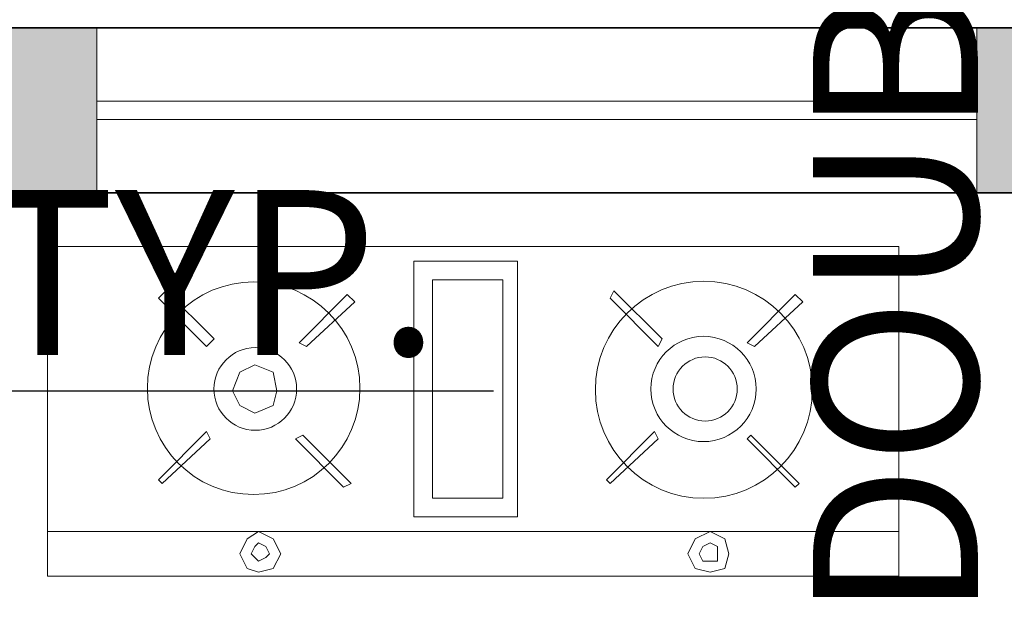
# Model space of a CAD drawing. Units: inches. Extents: x 2831 to 4250, y 1103 to 1797.
# Tile 9 of 15: x 3676 to 3730, y 1658 to 1690. Entities that reach past the tile are written whole.
import ezdxf

# ---------------------------------------------------------------- set-up
doc = ezdxf.new("R2010")
doc.units = ezdxf.units.IN
for name, color, linetype, lineweight in [('A-ANNO-DIMS', 2, 'Continuous', 18), ('A-EQPM', 8, 'Continuous', 18), ('A-WALL', 7, 'Continuous', 35), ('A-WALL-PATT', 252, 'Continuous', 13), ('window', 130, 'Continuous', 18)]:
    doc.layers.add(name, color=color, linetype=linetype, lineweight=lineweight)
doc.styles.get("Standard").update_dxf_attribs({"font": 'arial.ttf'})
doc.dimstyles.new('ISO-25', dxfattribs={"dimtxt": 9, "dimasz": 2.5, "dimexe": 1.25, "dimexo": 0.625, "dimtad": 1, "dimdec": 1, "dimlunit": 3, "dimtxsty": 'Standard', "dimcen": 2.5, "dimadec": 0, "dimazin": 0, "dimtfac": 1, "dimtdec": 1, "dimtmove": 0, "dimatfit": 3, "dimfxl": 1, "dimarcsym": 0})

# ---------------------------------------------------------------- blocks, each defined once
blk = doc.blocks.new('gas 1')
for points in [[(35.933, -1.875), (35.933, 0), (0, 0), (0, -1.875)], [(8.124, -0.937), (8.436, -1.562), (8.905, -1.875), (9.53, -1.562), (9.843, -0.937), (9.53, -0.312), (8.905, -0.156), (8.436, -0.312)], [(27.028, -0.937), (27.34, -1.562), (27.965, -1.875), (28.59, -1.562), (28.747, -0.937), (28.59, -0.312), (27.965, -0.156), (27.34, -0.312)], [(8.593, -0.937), (8.749, -1.25), (8.905, -1.406), (9.218, -1.25), (9.374, -0.937), (9.218, -0.781), (8.905, -0.625), (8.749, -0.781)], [(27.497, -0.937), (27.653, -1.25), (27.965, -1.406), (28.278, -1.25), (28.278, -0.937), (28.278, -0.625), (27.965, -0.625), (27.653, -0.625)], [(19.841, -13.28), (15.467, -13.28), (15.467, -2.5), (19.841, -2.5)], [(19.216, -12.498), (16.248, -12.498), (16.248, -3.281), (19.216, -3.281)], [(4.843, -3.906), (4.687, -4.062), (6.718, -6.093), (6.874, -5.781)], [(12.811, -3.906), (12.498, -3.75), (10.467, -5.781), (10.78, -5.937)], [(23.747, -3.906), (23.591, -4.062), (25.622, -6.093), (25.778, -5.781)], [(31.715, -3.906), (31.559, -3.75), (29.528, -5.781), (29.684, -5.937)], [(7.812, -7.812), (8.124, -8.593), (8.749, -8.905), (9.53, -8.593), (9.686, -7.812), (9.53, -7.187), (8.749, -6.874), (8.124, -7.187)], [(7.03, -9.999), (6.718, -9.686), (4.687, -11.717), (4.999, -12.03)], [(12.967, -11.561), (10.936, -9.686), (10.624, -9.843), (12.655, -11.874)], [(23.747, -11.717), (23.903, -12.03), (25.934, -9.999), (25.778, -9.686)], [(31.871, -11.561), (29.84, -9.686), (29.528, -9.843), (31.559, -11.874)]]:
    blk.add_lwpolyline(points, close=True)
blk.add_lwpolyline([(35.933, -1.875), (35.933, -13.905), (0, -13.905), (0, -1.875)])
for centre, radius in [((27.698, -7.857), 4.576), ((8.702, -7.922), 4.485), ((27.686, -7.89), 2.222), ((8.772, -7.89), 1.743), ((27.755, -7.89), 1.354)]:
    blk.add_circle(centre, radius)
blk = doc.blocks.new('WIN-48IN')
for p, q in [((9, 48), (0, 48)), ((4, 0), (4, 48)), ((5, 0), (5, 48)), ((9, 0), (0, 0))]:
    blk.add_line(p, q)
blk = doc.blocks.new('*D77')
at = {"layer": 'A-ANNO-DIMS', "color": 0, "lineweight": -2, "transparency": 16777216}
for p, q in [((3512.227, 1679.888), (3512.227, 1668.463)), ((3584.227, 1679.888), (3584.227, 1668.463)), ((3514.727, 1669.713), (3581.727, 1669.713)), ((3584.227, 1669.713), (3701.864, 1669.713))]:
    blk.add_line(p, q, dxfattribs=at)
at = {"layer": 'A-ANNO-DIMS', "color": 0, "transparency": 16777216}
for points in [[(3514.727, 1670.13), (3514.727, 1669.297), (3512.227, 1669.713)], [(3581.727, 1670.13), (3581.727, 1669.297), (3584.227, 1669.713)]]:
    blk.add_solid(points, dxfattribs=at)
at = {"layer": 'Defpoints', "color": 0, "transparency": 16777216}
for p in [(3512.227, 1680.513), (3584.227, 1680.513), (3584.227, 1669.713)]:
    blk.add_point(p, dxfattribs=at)
at = {"layer": 'A-ANNO-DIMS', "color": 0, "transparency": 16777216, "insert": (3644.295, 1674.995), "char_height": 9, "attachment_point": 5}
blk.add_mtext('WINDOW 6\'-0" TYP.', dxfattribs=at)
blk = doc.blocks.new('*D85')
at = {"layer": 'A-ANNO-DIMS', "color": 0, "lineweight": -2, "transparency": 16777216}
for p, q in [((3730.24, 1651.147), (3730.24, 1797.343)), ((3735.015, 1651.147), (3728.99, 1651.147)), ((3730.24, 1617.647), (3730.24, 1648.647)), ((3735.015, 1615.147), (3728.99, 1615.147))]:
    blk.add_line(p, q, dxfattribs=at)
at = {"layer": 'A-ANNO-DIMS', "color": 0, "transparency": 16777216}
for points in [[(3729.823, 1648.647), (3730.657, 1648.647), (3730.24, 1651.147)], [(3729.823, 1617.647), (3730.657, 1617.647), (3730.24, 1615.147)]]:
    blk.add_solid(points, dxfattribs=at)
at = {"layer": 'Defpoints', "color": 0, "transparency": 16777216}
for p in [(3730.24, 1651.147), (3735.64, 1651.147), (3735.64, 1615.147)]:
    blk.add_point(p, dxfattribs=at)
at = {"layer": 'A-ANNO-DIMS', "color": 0, "transparency": 16777216, "insert": (3724.955, 1725.495), "char_height": 9, "attachment_point": 5, "rotation": 90}
blk.add_mtext('DOUBLE SINK 3\'-0" TYP.', dxfattribs=at)

msp = doc.modelspace()

# ---------------------------------------------------------------- hatches: boundary and pattern name
at = {"layer": 'A-WALL-PATT'}
h = msp.add_hatch(color=256, dxfattribs=at)
h.dxf.hatch_style = 1
h.paths.add_polyline_path([(3783.227, 1560.513), (3767.227, 1560.513), (3767.227, 1572.513), (3761.227, 1572.513), (3758.227, 1572.513), (3758.227, 1560.513), (3488.227, 1560.513), (3488.227, 1562.513), (3485.227, 1562.513), (3479.227, 1562.513), (3479.227, 1552.513), (3485.227, 1552.513), (3488.227, 1552.513), (3488.227, 1554.513), (3642.227, 1554.513), (3642.227, 1498.513), (3648.227, 1498.513), (3648.227, 1554.513), (3720.227, 1554.513), (3720.227, 1498.513), (3726.227, 1498.513), (3726.227, 1554.513), (3774.227, 1554.513), (3774.227, 1528.513), (3783.227, 1528.513)])
h.paths.add_polyline_path([(3767.227, 1689.513), (3728.227, 1689.513), (3728.227, 1680.513), (3758.227, 1680.513), (3758.227, 1602.513), (3767.227, 1602.513)])
h.paths.add_polyline_path([(3680.227, 1689.513), (3656.227, 1689.513), (3656.227, 1680.513), (3662.227, 1680.513), (3662.227, 1608.513), (3644.227, 1608.513), (3644.227, 1602.513), (3668.227, 1602.513), (3668.227, 1680.513), (3680.227, 1680.513)])
h.paths.add_polyline_path([(3620.227, 1689.513), (3584.227, 1689.513), (3584.227, 1680.513), (3608.227, 1680.513), (3608.227, 1602.513), (3614.227, 1602.513), (3614.227, 1608.513), (3614.227, 1638.513), (3614.227, 1680.513), (3620.227, 1680.513)])
h.paths.add_polyline_path([(3512.227, 1689.513), (3479.227, 1689.513), (3479.227, 1665.513), (3488.227, 1665.513), (3488.227, 1680.513), (3512.227, 1680.513)])
h.paths.add_polyline_path([(3488.227, 1617.513), (3479.227, 1617.513), (3479.227, 1602.513), (3485.227, 1602.513), (3488.227, 1602.513)])

# ---------------------------------------------------------------- linework, layer by layer
at = {"layer": 'A-WALL'}
for p, q in [((3479.227, 1689.513), (3803.227, 1689.513)), ((3668.227, 1680.513), (3758.227, 1680.513))]:
    msp.add_line(p, q, dxfattribs=at)

# ---------------------------------------------------------------- block references
at = {"layer": 'A-EQPM', "xscale": -1.292580420916565, "yscale": 1.292580420916565, "zscale": 1.292580420916565, "rotation": 180}
msp.add_blockref('gas 1', (3677.535, 1659.616), dxfattribs=at)
at = {"layer": 'window', "rotation": 90}
msp.add_blockref('WIN-48IN', (3728.227, 1680.513), dxfattribs=at)

# ---------------------------------------------------------------- dimensions: what is measured, and where the dimension line sits
at = {"layer": 'A-ANNO-DIMS'}
dim = msp.add_linear_dim(base=(3730.24, 1651.147), p1=(3735.64, 1615.147), p2=(3735.64, 1651.147), angle=90, text='DOUBLE SINK <> TYP.', dimstyle='ISO-25', override={"dimdec": 1, "dimlfac": 1, "dimrnd": 0, "dimzin": 1, "dimdsep": 46, "dimlunit": 4, "dimfrac": 2}, dxfattribs=at)
dim.commit()
dim.dimension.update_dxf_attribs({"geometry": '*D85', "text_midpoint": (3724.955, 1725.495)})
dim = msp.add_linear_dim(base=(3584.227, 1669.713), p1=(3512.227, 1680.513), p2=(3584.227, 1680.513), text='WINDOW <> TYP.', dimstyle='ISO-25', override={"dimdec": 1, "dimlfac": 1, "dimrnd": 0, "dimzin": 1, "dimdsep": 46, "dimlunit": 4, "dimfrac": 2}, dxfattribs=at)
dim.commit()
dim.dimension.update_dxf_attribs({"geometry": '*D77', "text_midpoint": (3644.295, 1674.995)})

doc.saveas('drawing.dxf')
